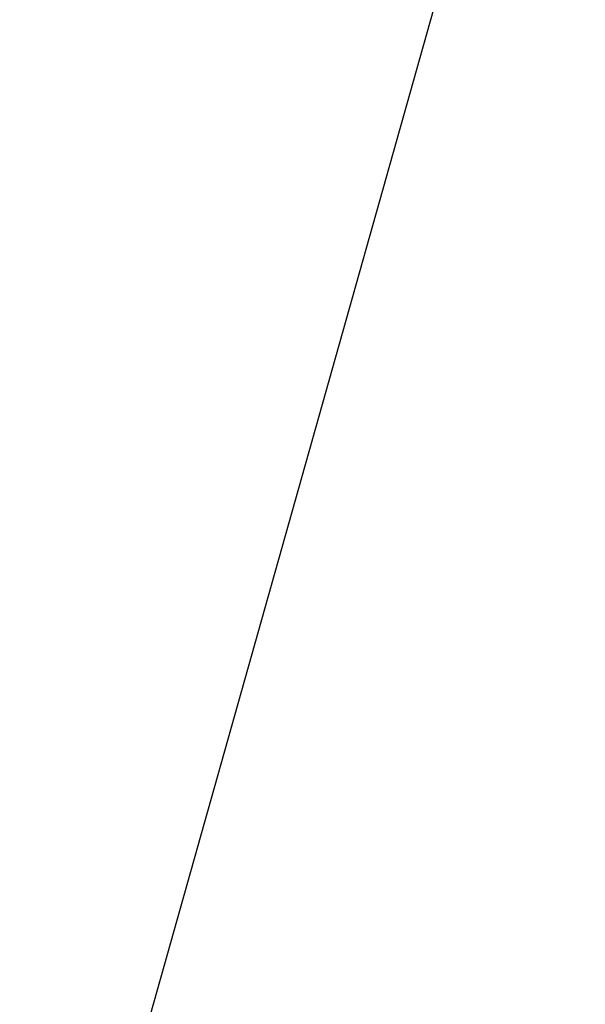
# Model space of a CAD drawing. Units: inches. Extents: x 3590 to 5167, y 65 to 1917.
# Tile 88 of 100: x 5052.5773 to 5052.8768, y 1788.0928 to 1788.6144. Entities that reach past the tile are written whole.
import ezdxf

# ---------------------------------------------------------------- set-up
doc = ezdxf.new("R2010")
doc.units = ezdxf.units.IN
for name, color, linetype, lineweight in [('A-ANNO-DIMS', 2, 'Continuous', 18), ('A-FLOR-PATT', 8, 'Continuous', 13), ('L-PLNT', 94, 'Continuous', 18)]:
    doc.layers.add(name, color=color, linetype=linetype, lineweight=lineweight)
doc.layers.add('DIENHOA', color=3, linetype='Continuous')
doc.styles.get("Standard").update_dxf_attribs({"font": 'arial.ttf'})
doc.dimstyles.new('ISO-25', dxfattribs={"dimtxt": 9, "dimasz": 2.5, "dimexe": 1.25, "dimexo": 0.625, "dimtad": 1, "dimdec": 1, "dimlunit": 3, "dimtxsty": 'Standard', "dimcen": 2.5, "dimadec": 0, "dimazin": 0, "dimtfac": 1, "dimtdec": 1, "dimtmove": 0, "dimatfit": 3, "dimfxl": 1, "dimarcsym": 0})

# ---------------------------------------------------------------- blocks, each defined once
blk = doc.blocks.new('Cay03_mb')
at = {"layer": 'DIENHOA'}
blk.add_line((96.72, 365.576), (75.598, 290.611), dxfattribs=at)
blk = doc.blocks.new('*D322')
at = {"layer": 'A-ANNO-DIMS', "color": 0, "lineweight": -2, "transparency": 16777216}
for p, q in [((5035.74373, 1766.18424), (5035.74373, 1761.19899)), ((5064.81203, 1766.18424), (5064.81203, 1761.19899)), ((5038.24373, 1762.44899), (5062.31203, 1762.44899)), ((5064.81203, 1762.44899), (5166.99109, 1762.44899))]:
    blk.add_line(p, q, dxfattribs=at)
at = {"layer": 'A-ANNO-DIMS', "color": 0, "transparency": 16777216}
for points in [[(5038.24373, 1762.86566), (5038.24373, 1762.03233), (5035.74373, 1762.44899)], [(5062.31203, 1762.86566), (5062.31203, 1762.03233), (5064.81203, 1762.44899)]]:
    blk.add_solid(points, dxfattribs=at)
at = {"layer": 'Defpoints', "color": 0, "transparency": 16777216}
for p in [(5035.74373, 1766.80924), (5064.81203, 1766.80924), (5064.81203, 1762.44899)]:
    blk.add_point(p, dxfattribs=at)
at = {"layer": 'A-ANNO-DIMS', "color": 0, "transparency": 16777216, "insert": (5117.15156, 1767.66915), "char_height": 9, "attachment_point": 5}
blk.add_mtext('PLANT 2\'-5" TYP.', dxfattribs=at)

msp = doc.modelspace()

# ---------------------------------------------------------------- hatches: boundary and pattern name
at = {"layer": 'A-FLOR-PATT', "transparency": 33554687}
h = msp.add_hatch(dxfattribs=at)
h.set_pattern_fill('AR-HBONE', color=256, scale=0.2)
h.set_pattern_definition([(45, (-588.972, 0), (0, 28.73682), [60.96, -20.32]), (135, (-574.604, 14.368), (3e-15, 28.73682), [60.96, -20.32])])
h.paths.add_polyline_path([(5071.27403, 1796.99898), (4933.27403, 1796.99898), (4933.27403, 1753.99898), (4962.77403, 1753.99898, -0.414214), (4928.77403, 1719.99898), (4933.27403, 1718.99898), (4933.27403, 1334.99898), (5071.27403, 1334.99898)])
h.paths.add_polyline_path([(4951.78002, 1521.0767), (4951.7151, 1521.0404), (4951.56345, 1520.89532)], flags=16)
h.paths.add_polyline_path([(4952.267, 1521.37645), (4952.1977, 1521.37111), (4952.19823, 1521.35558)], flags=0)
h.paths.add_polyline_path([(4967.05076, 1529.72832), (4965.23122, 1528.69444), (4963.41109, 1527.71401), (4961.75649, 1526.85081), (4963.58887, 1527.44938), (4964.03555, 1527.47802), (4962.9755, 1527.24902), (4961.76022, 1526.85203), (4959.79219, 1525.83406), (4958.00498, 1524.89483), (4956.24031, 1523.92961), (4954.50395, 1522.91854), (4954.1294, 1522.68163), (4953.36051, 1521.99688), (4953.36558, 1521.99754), (4953.605, 1522.06367), (4955.10605, 1522.76083), (4956.92108, 1523.43405), (4958.67784, 1523.91513), (4960.35834, 1524.20036), (4961.94456, 1524.28606), (4964.17144, 1524.10849), (4965.95752, 1523.30903), (4963.86273, 1522.97565), (4965.18742, 1522.49898), (4963.36614, 1522.49715), (4961.54526, 1522.48682), (4959.76359, 1522.46077), (4958.30414, 1522.4188), (4957.97356, 1522.38829), (4956.30692, 1522.2324), (4954.71821, 1522.07143), (4953.25077, 1521.89915), (4953.52509, 1521.62277), (4954.33087, 1521.37883), (4956.24263, 1521.22987), (4958.03913, 1520.92952), (4959.68424, 1520.48339), (4961.16007, 1519.89569), (4963.10699, 1518.80022), (4964.39286, 1517.32518), (4962.97306, 1517.72596), (4964.55841, 1516.66059), (4965.40664, 1515.70779), (4963.50733, 1516.32179), (4961.67995, 1517.0051), (4959.93478, 1517.74489), (4958.2821, 1518.52833), (4956.73216, 1519.34257), (4955.29527, 1520.17478), (4954.67155, 1520.57237), (4954.51279, 1520.6271), (4955.65848, 1519.31837), (4956.70263, 1517.98232), (4957.64403, 1516.64663), (4958.48545, 1515.33439), (4959.54998, 1513.52398), (4960.43768, 1511.76936), (4958.84107, 1513.6196), (4957.45175, 1515.3249), (4955.8186, 1517.45855), (4956.66537, 1515.44764), (4957.11109, 1513.92292), (4957.44681, 1511.71434), (4957.07641, 1509.79288), (4956.53757, 1511.1103), (4955.99231, 1512.56892), (4955.44448, 1514.12509), (4954.89794, 1515.73518), (4954.35653, 1517.35553), (4953.82412, 1518.94251), (4953.30455, 1520.45247), (4953.06452, 1521.11563), (4952.97143, 1521.14607), (4952.94932, 1521.08646), (4952.72981, 1520.19905), (4953.3698, 1518.02364), (4953.75708, 1516.37279), (4954.05124, 1514.76538), (4954.26449, 1513.22121), (4954.47124, 1511.13121), (4954.4971, 1510.40174), (4954.40903, 1511.76006), (4954.26449, 1513.22121), (4954.05124, 1514.76538), (4953.75708, 1516.37279), (4953.3698, 1518.02364), (4952.87718, 1519.69813), (4952.7161, 1520.1412), (4952.53301, 1519.05871), (4952.37428, 1517.78881), (4952.21925, 1516.31167), (4952.04598, 1514.59986), (4951.83253, 1512.62598), (4951.55697, 1510.36259), (4951.20331, 1512.16818), (4950.85168, 1514.33931), (4950.98529, 1516.37594), (4951.6596, 1518.28625), (4952.59261, 1520.48085), (4952.35664, 1521.1299), (4951.85502, 1520.32753), (4950.83901, 1518.90828), (4949.77675, 1517.58658), (4948.91554, 1516.61731), (4948.11099, 1515.2561), (4947.0891, 1513.55389), (4945.88937, 1511.61495), (4946.32587, 1513.40232), (4946.5624, 1514.24913), (4945.52771, 1513.32668), (4944.58105, 1512.53126), (4946.01774, 1514.50825), (4947.2044, 1516.04763), (4947.89331, 1517.31331), (4949.30686, 1518.76446), (4950.41417, 1519.76716), (4950.45131, 1519.80628), (4952.267, 1521.37645), (4951.64457, 1521.49317), (4950.40371, 1521.17954), (4948.04447, 1520.35868), (4946.11863, 1519.45198), (4944.57182, 1518.47484), (4943.34962, 1517.44265), (4941.99695, 1515.91971), (4941.66146, 1515.27475), (4942.81332, 1516.98973), (4944.57182, 1518.47484), (4946.11863, 1519.45198), (4948.04447, 1520.35868), (4950.40371, 1521.17954), (4951.64457, 1521.49317), (4949.64678, 1521.86781), (4948.59979, 1521.75633), (4947.12629, 1521.5699), (4945.42015, 1521.34763), (4943.44969, 1521.10462), (4941.18319, 1520.85596), (4942.86028, 1521.61265), (4943.87308, 1522.03014), (4942.95216, 1521.9093), (4941.40968, 1521.48512), (4939.54287, 1520.67019), (4938.96775, 1520.2255), (4940.73284, 1521.29899), (4942.95216, 1521.9093), (4943.70184, 1522.00767), (4945.89419, 1522.69998), (4947.56488, 1522.71399), (4948.92086, 1522.56573), (4951.13144, 1522.18271), (4950.97062, 1522.2969), (4948.12924, 1523.00563), (4946.03496, 1523.70671), (4944.23235, 1524.52143), (4942.70692, 1525.46111), (4941.44419, 1526.53707), (4940.42968, 1527.76062), (4939.6489, 1529.14306), (4941.42091, 1528.12232), (4943.14742, 1527.13248), (4944.84093, 1526.17457), (4946.51394, 1525.24959), (4948.17893, 1524.35855), (4948.36457, 1524.26336), (4946.47531, 1526.04459), (4945.18083, 1527.54042), (4944.19039, 1529.03339), (4943.49559, 1530.53985), (4943.27808, 1531.3597), (4942.49849, 1531.91903), (4943.11353, 1531.76249), (4942.95927, 1533.6586), (4944.13953, 1531.9886), (4944.61171, 1531.32339), (4946.20163, 1530.46341), (4947.48567, 1529.50925), (4948.79027, 1528.22649), (4950.36754, 1526.23746), (4949.48547, 1528.15549), (4948.85128, 1530.12254), (4948.49054, 1532.04127), (4948.38105, 1533.91822), (4948.50062, 1535.7599), (4948.82704, 1537.57284), (4949.41803, 1535.56526), (4949.95684, 1533.56932), (4950.46414, 1531.5861), (4950.96058, 1529.6167), (4951.3911, 1527.95448), (4951.72352, 1530.68689), (4952.20106, 1532.57994), (4952.88914, 1534.32964), (4953.77035, 1535.95123), (4954.82726, 1537.45995), (4954.52145, 1535.38966), (4954.27314, 1533.93684), (4955.57999, 1535.6627), (4956.74758, 1536.73859), (4956.15852, 1534.78029), (4955.58917, 1532.87334), (4955.04336, 1531.00581), (4954.52493, 1529.16576), (4954.03771, 1527.34127), (4953.63833, 1525.73298), (4953.61143, 1525.58564), (4953.39805, 1524.16565), (4953.38219, 1524.00887), (4954.06955, 1525.47563), (4954.91212, 1527.02173), (4956.13627, 1528.89351), (4957.84668, 1530.57701), (4959.37601, 1531.54014), (4958.25596, 1530.10398), (4957.14284, 1528.66291), (4956.06626, 1527.24305), (4955.05579, 1525.87054), (4954.14104, 1524.57149), (4953.35159, 1523.37204), (4953.31079, 1523.30299), (4953.27253, 1522.92478), (4953.26102, 1522.38213), (4954.1031, 1523.37273), (4954.63005, 1524.28376), (4955.96149, 1526.35767), (4957.23002, 1528.12969), (4958.42057, 1529.60864), (4960.03671, 1531.36792), (4961.3736, 1532.3752), (4962.1015, 1532.77), (4961.06994, 1531.06113), (4959.98733, 1529.43811), (4958.86851, 1527.90803), (4958.15046, 1527.00742), (4959.80291, 1528.00314), (4961.58854, 1528.79257), (4963.39087, 1529.32783), (4965.21118, 1529.63205)], flags=16)
h.paths.add_polyline_path([(4962.94387, 1523.18187), (4961.10714, 1523.42192), (4960.39205, 1523.36158), (4962.34964, 1523.33061)], flags=0)
h.paths.add_polyline_path([(5049.54129, 1584.55089), (5049.47636, 1584.51458), (5049.32471, 1584.3695)], flags=16)
h.paths.add_polyline_path([(5050.02827, 1584.85063), (5049.95897, 1584.84529), (5049.95949, 1584.82976)], flags=0)
h.paths.add_polyline_path([(5042.33308, 1581.94902), (5043.8799, 1582.92616), (5045.80573, 1583.83286), (5048.16498, 1584.65372), (5049.40583, 1584.96736), (5047.40804, 1585.34199), (5046.36106, 1585.23052), (5044.88755, 1585.04408), (5043.18142, 1584.82181), (5041.21095, 1584.5788), (5038.94446, 1584.33014), (5040.62155, 1585.08683), (5041.63434, 1585.50432), (5040.71343, 1585.38348), (5039.17095, 1584.9593), (5037.30414, 1584.14438), (5036.72901, 1583.69969), (5038.4941, 1584.77317), (5040.71343, 1585.38348), (5041.4631, 1585.48185), (5043.65545, 1586.17416), (5045.32615, 1586.18818), (5046.68212, 1586.03992), (5048.8927, 1585.6569), (5048.73188, 1585.77108), (5045.89051, 1586.47981), (5043.79622, 1587.18089), (5041.99361, 1587.99561), (5040.46818, 1588.9353), (5039.20546, 1590.01125), (5038.19095, 1591.2348), (5037.41016, 1592.61725), (5039.18217, 1591.5965), (5040.90868, 1590.60667), (5042.6022, 1589.64876), (5044.2752, 1588.72378), (5045.94019, 1587.83274), (5046.12584, 1587.73754), (5044.23658, 1589.51878), (5042.9421, 1591.01461), (5041.95166, 1592.50757), (5041.25685, 1594.01403), (5041.03935, 1594.83388), (5040.25976, 1595.39321), (5040.8748, 1595.23667), (5040.72054, 1597.13279), (5041.9008, 1595.46278), (5042.37297, 1594.79758), (5043.96289, 1593.93759), (5045.24694, 1592.98344), (5046.55153, 1591.70068), (5048.12881, 1589.71164), (5047.24673, 1591.62967), (5046.61254, 1593.59672), (5046.2518, 1595.51546), (5046.14232, 1597.3924), (5046.26189, 1599.23408), (5046.5883, 1601.04703), (5047.17929, 1599.03944), (5047.71811, 1597.0435), (5048.22541, 1595.06028), (5048.72184, 1593.09089), (5049.15237, 1591.42866), (5049.48478, 1594.16107), (5049.96233, 1596.05412), (5050.65041, 1597.80382), (5051.53161, 1599.42541), (5052.58852, 1600.93414), (5052.28271, 1598.86384), (5052.03441, 1597.41102), (5053.34126, 1599.13689), (5054.50884, 1600.21277), (5053.91979, 1598.25447), (5053.35044, 1596.34752), (5052.80463, 1594.47999), (5052.2862, 1592.63995), (5051.79898, 1590.81546), (5051.39959, 1589.20716), (5051.3727, 1589.05983), (5051.15931, 1587.63984), (5051.14346, 1587.48305), (5051.83082, 1588.94982), (5052.67339, 1590.49592), (5053.89754, 1592.3677), (5055.60794, 1594.05119), (5057.13728, 1595.01432), (5056.01722, 1593.57817), (5054.90411, 1592.1371), (5053.82752, 1590.71724), (5052.81705, 1589.34472), (5051.9023, 1588.04567), (5051.11286, 1586.84622), (5051.07205, 1586.77718), (5051.03379, 1586.39896), (5051.02228, 1585.85631), (5051.86437, 1586.84692), (5052.39131, 1587.75794), (5053.72275, 1589.83185), (5054.99128, 1591.60387), (5056.18183, 1593.08282), (5057.79798, 1594.84211), (5059.13486, 1595.84938), (5059.86276, 1596.24419), (5058.83121, 1594.53531), (5057.7486, 1592.9123), (5056.62978, 1591.38221), (5055.91173, 1590.4816), (5057.56418, 1591.47732), (5059.34981, 1592.26675), (5061.15214, 1592.80202), (5062.97245, 1593.10624), (5064.81203, 1593.20251), (5062.99248, 1592.16863), (5061.17235, 1591.18819), (5059.51775, 1590.325), (5061.35014, 1590.92356), (5061.79682, 1590.95221), (5060.73676, 1590.7232), (5059.52148, 1590.32622), (5057.55345, 1589.30825), (5055.76625, 1588.36901), (5054.00157, 1587.40379), (5052.26521, 1586.39273), (5051.89067, 1586.15581), (5051.12177, 1585.47106), (5051.12684, 1585.47172), (5051.36627, 1585.53786), (5052.86732, 1586.23502), (5054.68234, 1586.90824), (5056.4391, 1587.38931), (5058.1196, 1587.67454), (5059.70582, 1587.76024), (5061.93271, 1587.58268), (5063.71878, 1586.78321), (5061.62399, 1586.44983), (5062.94869, 1585.97317), (5061.12741, 1585.97133), (5059.30653, 1585.961), (5057.52486, 1585.93496), (5056.06541, 1585.89299), (5055.73482, 1585.86247), (5054.06819, 1585.70658), (5052.47947, 1585.54561), (5051.01204, 1585.37333), (5051.28635, 1585.09695), (5052.09214, 1584.85301), (5054.00389, 1584.70406), (5055.8004, 1584.4037), (5057.44551, 1583.95757), (5058.92133, 1583.36987), (5060.86825, 1582.27441), (5062.15413, 1580.79937), (5060.73433, 1581.20015), (5062.31967, 1580.13477), (5063.1679, 1579.18198), (5061.2686, 1579.79597), (5059.44122, 1580.47928), (5057.69605, 1581.21908), (5056.04336, 1582.00251), (5054.49343, 1582.81675), (5053.05653, 1583.64897), (5052.43281, 1584.04656), (5052.27405, 1584.10128), (5053.41974, 1582.79255), (5054.4639, 1581.4565), (5055.40529, 1580.12081), (5056.24672, 1578.80858), (5057.31125, 1576.99816), (5058.19895, 1575.24354), (5056.60234, 1577.09378), (5055.21301, 1578.79908), (5053.57987, 1580.93274), (5054.42664, 1578.92183), (5054.87235, 1577.3971), (5055.20808, 1575.18852), (5054.83767, 1573.26706), (5054.29883, 1574.58448), (5053.75357, 1576.0431), (5053.20575, 1577.59927), (5052.6592, 1579.20936), (5052.1178, 1580.82971), (5051.58538, 1582.41669), (5051.06582, 1583.92666), (5050.82578, 1584.58981), (5050.7327, 1584.62025), (5050.71058, 1584.56064), (5050.49108, 1583.67323), (5051.13107, 1581.49782), (5051.51835, 1579.84698), (5051.8125, 1578.23957), (5052.02575, 1576.69539), (5052.23251, 1574.6054), (5052.25836, 1573.87593), (5052.1703, 1575.23424), (5052.02575, 1576.69539), (5051.8125, 1578.23957), (5051.51835, 1579.84698), (5051.13107, 1581.49782), (5050.63844, 1583.17231), (5050.47736, 1583.61538), (5050.29428, 1582.53289), (5050.13554, 1581.26299), (5049.98051, 1579.78585), (5049.80724, 1578.07405), (5049.59379, 1576.10016), (5049.31823, 1573.83678), (5048.96458, 1575.64237), (5048.61294, 1577.8135), (5048.74656, 1579.85012), (5049.42086, 1581.76043), (5050.35388, 1583.95503), (5050.1179, 1584.60408), (5049.61629, 1583.80172), (5048.60027, 1582.38246), (5047.53801, 1581.06076), (5046.67681, 1580.09149), (5045.87225, 1578.73029), (5044.85036, 1577.02808), (5043.65063, 1575.08913), (5044.08713, 1576.8765), (5044.32366, 1577.72331), (5043.28898, 1576.80086), (5042.34232, 1576.00545), (5043.779, 1577.98243), (5044.96566, 1579.52182), (5045.65457, 1580.78749), (5047.06813, 1582.23865), (5048.17543, 1583.24134), (5048.21258, 1583.28047), (5050.02827, 1584.85063), (5049.40583, 1584.96736), (5048.16498, 1584.65372), (5045.80573, 1583.83286), (5043.8799, 1582.92616), (5042.33308, 1581.94902), (5041.11088, 1580.91684), (5039.75821, 1579.39389), (5039.42272, 1578.74894), (5040.57458, 1580.46391)], flags=16)
h.paths.add_polyline_path([(4954.79872, 1533.12029), (4954.26249, 1532.07935), (4953.83112, 1530.93464), (4953.50472, 1529.63602), (4953.28338, 1528.13331), (4953.16721, 1526.37637), (4953.15631, 1524.31504), (4953.27669, 1521.23629), (4952.80168, 1521.84177), (4951.55695, 1521.99789), (4950.97575, 1521.9613), (4952.66059, 1521.94097), (4952.80168, 1521.84177), (4953.15249, 1523.59258), (4953.16721, 1526.37637), (4953.28338, 1528.13331), (4953.60929, 1530.34598), (4954.45558, 1532.59174)], flags=0)
h.paths.add_polyline_path([(5050.56294, 1585.31596), (5049.31822, 1585.47208), (5048.73702, 1585.43548), (5050.42186, 1585.41516), (5050.56294, 1585.31596), (5050.91375, 1587.06676), (5050.92848, 1589.85056), (5051.04465, 1591.6075), (5051.37055, 1593.82017), (5052.21684, 1596.06593), (5052.55999, 1596.59447), (5052.02375, 1595.55353), (5051.59238, 1594.40883), (5051.26598, 1593.1102), (5051.04465, 1591.6075), (5050.92848, 1589.85056), (5050.91757, 1587.78922), (5051.03795, 1584.71048)], flags=0)
h.paths.add_polyline_path([(5058.15332, 1586.83576), (5060.11091, 1586.80479), (5060.70514, 1586.65605), (5058.8684, 1586.8961)], flags=0)
h.paths.add_polyline_path([(5049.54129, 1430.93611), (5049.47636, 1430.8998), (5049.32471, 1430.75472)], flags=16)
h.paths.add_polyline_path([(5050.02827, 1431.23585), (5049.95897, 1431.23051), (5049.95949, 1431.21498)], flags=0)
h.paths.add_polyline_path([(5046.5883, 1447.43225), (5047.17929, 1445.42467), (5047.71811, 1443.42872), (5048.22541, 1441.4455), (5048.72184, 1439.47611), (5049.15237, 1437.81388), (5049.48478, 1440.5463), (5049.96233, 1442.43934), (5050.65041, 1444.18904), (5051.53161, 1445.81063), (5052.58852, 1447.31936), (5052.28271, 1445.24906), (5052.03441, 1443.79624), (5053.34126, 1445.52211), (5054.50884, 1446.59799), (5053.91979, 1444.63969), (5053.35044, 1442.73274), (5052.80463, 1440.86521), (5052.2862, 1439.02517), (5051.79898, 1437.20068), (5051.39959, 1435.59238), (5051.3727, 1435.44505), (5051.15931, 1434.02506), (5051.14346, 1433.86828), (5051.83082, 1435.33504), (5052.67339, 1436.88114), (5053.89754, 1438.75292), (5055.60794, 1440.43641), (5057.13728, 1441.39954), (5056.01722, 1439.96339), (5054.90411, 1438.52232), (5053.82752, 1437.10246), (5052.81705, 1435.72994), (5051.9023, 1434.4309), (5051.11286, 1433.23145), (5051.07205, 1433.1624), (5051.03379, 1432.78418), (5051.02228, 1432.24153), (5051.86437, 1433.23214), (5052.39131, 1434.14316), (5053.72275, 1436.21707), (5054.99128, 1437.98909), (5056.18183, 1439.46805), (5057.79798, 1441.22733), (5059.13486, 1442.23461), (5059.86276, 1442.62941), (5058.83121, 1440.92053), (5057.7486, 1439.29752), (5056.62978, 1437.76743), (5055.91173, 1436.86682), (5057.56418, 1437.86255), (5059.34981, 1438.65197), (5061.15214, 1439.18724), (5062.97245, 1439.49146), (5064.81203, 1439.58773), (5062.99248, 1438.55385), (5061.17235, 1437.57342), (5059.51775, 1436.71022), (5061.35014, 1437.30879), (5061.79682, 1437.33743), (5060.73676, 1437.10842), (5059.52148, 1436.71144), (5057.55345, 1435.69347), (5055.76625, 1434.75423), (5054.00157, 1433.78901), (5052.26521, 1432.77795), (5051.89067, 1432.54103), (5051.12177, 1431.85628), (5051.12684, 1431.85694), (5051.36627, 1431.92308), (5052.86732, 1432.62024), (5054.68234, 1433.29346), (5056.4391, 1433.77453), (5058.1196, 1434.05976), (5059.70582, 1434.14546), (5061.93271, 1433.9679), (5063.71878, 1433.16843), (5061.62399, 1432.83505), (5062.94869, 1432.35839), (5061.12741, 1432.35655), (5059.30653, 1432.34623), (5057.52486, 1432.32018), (5056.06541, 1432.27821), (5055.73482, 1432.24769), (5054.06819, 1432.09181), (5052.47947, 1431.93083), (5051.01204, 1431.75856), (5051.28635, 1431.48218), (5052.09214, 1431.23823), (5054.00389, 1431.08928), (5055.8004, 1430.78892), (5057.44551, 1430.34279), (5058.92133, 1429.75509), (5060.86825, 1428.65963), (5062.15413, 1427.18459), (5060.73433, 1427.58537), (5062.31967, 1426.52), (5063.1679, 1425.5672), (5061.2686, 1426.18119), (5059.44122, 1426.86451), (5057.69605, 1427.6043), (5056.04336, 1428.38773), (5054.49343, 1429.20197), (5053.05653, 1430.03419), (5052.43281, 1430.43178), (5052.27405, 1430.48651), (5053.41974, 1429.17777), (5054.4639, 1427.84172), (5055.40529, 1426.50603), (5056.24672, 1425.1938), (5057.31125, 1423.38338), (5058.19895, 1421.62877), (5056.60234, 1423.479), (5055.21301, 1425.1843), (5053.57987, 1427.31796), (5054.42664, 1425.30705), (5054.87235, 1423.78233), (5055.20808, 1421.57374), (5054.83767, 1419.65228), (5054.29883, 1420.9697), (5053.75357, 1422.42832), (5053.20575, 1423.9845), (5052.6592, 1425.59458), (5052.1178, 1427.21493), (5051.58538, 1428.80191), (5051.06582, 1430.31188), (5050.82578, 1430.97503), (5050.7327, 1431.00547), (5050.71058, 1430.94586), (5050.49108, 1430.05845), (5051.13107, 1427.88305), (5051.51835, 1426.2322), (5051.8125, 1424.62479), (5052.02575, 1423.08061), (5052.23251, 1420.99062), (5052.25836, 1420.26115), (5052.1703, 1421.61947), (5052.02575, 1423.08061), (5051.8125, 1424.62479), (5051.51835, 1426.2322), (5051.13107, 1427.88305), (5050.63844, 1429.55753), (5050.47736, 1430.0006), (5050.29428, 1428.91811), (5050.13554, 1427.64821), (5049.98051, 1426.17107), (5049.80724, 1424.45927), (5049.59379, 1422.48539), (5049.31823, 1420.222), (5048.96458, 1422.02759), (5048.61294, 1424.19872), (5048.74656, 1426.23534), (5049.42086, 1428.14565), (5050.35388, 1430.34025), (5050.1179, 1430.98931), (5049.61629, 1430.18694), (5048.60027, 1428.76768), (5047.53801, 1427.44598), (5046.67681, 1426.47671), (5045.87225, 1425.11551), (5044.85036, 1423.4133), (5043.65063, 1421.47435), (5044.08713, 1423.26172), (5044.32366, 1424.10854), (5043.28898, 1423.18608), (5042.34232, 1422.39067), (5043.779, 1424.36765), (5044.96566, 1425.90704), (5045.65457, 1427.17272), (5047.06813, 1428.62387), (5048.17543, 1429.62657), (5048.21258, 1429.66569), (5050.02827, 1431.23585), (5049.40583, 1431.35258), (5048.16498, 1431.03894), (5045.80573, 1430.21809), (5043.8799, 1429.31139), (5042.33308, 1428.33424), (5041.11088, 1427.30206), (5039.75821, 1425.77911), (5039.42272, 1425.13416), (5040.57458, 1426.84914), (5042.33308, 1428.33424), (5043.8799, 1429.31139), (5045.80573, 1430.21809), (5048.16498, 1431.03894), (5049.40583, 1431.35258), (5047.40804, 1431.72722), (5046.36106, 1431.61574), (5044.88755, 1431.42931), (5043.18142, 1431.20704), (5041.21095, 1430.96402), (5038.94446, 1430.71536), (5040.62155, 1431.47205), (5041.63434, 1431.88954), (5040.71343, 1431.76871), (5039.17095, 1431.34453), (5037.30414, 1430.5296), (5036.72901, 1430.08491), (5038.4941, 1431.1584), (5040.71343, 1431.76871), (5041.4631, 1431.86707), (5043.65545, 1432.55939), (5045.32615, 1432.5734), (5046.68212, 1432.42514), (5048.8927, 1432.04212), (5048.73188, 1432.1563), (5045.89051, 1432.86503), (5043.79622, 1433.56611), (5041.99361, 1434.38083), (5040.46818, 1435.32052), (5039.20546, 1436.39648), (5038.19095, 1437.62002), (5037.41016, 1439.00247), (5039.18217, 1437.98172), (5040.90868, 1436.99189), (5042.6022, 1436.03398), (5044.2752, 1435.109), (5045.94019, 1434.21796), (5046.12584, 1434.12276), (5044.23658, 1435.904), (5042.9421, 1437.39983), (5041.95166, 1438.8928), (5041.25685, 1440.39925), (5041.03935, 1441.2191), (5040.25976, 1441.77844), (5040.8748, 1441.62189), (5040.72054, 1443.51801), (5041.9008, 1441.848), (5042.37297, 1441.1828), (5043.96289, 1440.32282), (5045.24694, 1439.36866), (5046.55153, 1438.0859), (5048.12881, 1436.09686), (5047.24673, 1438.01489), (5046.61254, 1439.98195), (5046.2518, 1441.90068), (5046.14232, 1443.77762), (5046.26189, 1445.6193)], flags=16)
h.paths.add_polyline_path([(5052.38176, 1444.25496), (5051.62263, 1442.77987), (5052.02375, 1441.93875), (5052.55999, 1442.9797)], flags=0)
h.paths.add_polyline_path([(5050.56294, 1431.70118), (5049.31822, 1431.8573), (5048.73702, 1431.82071), (5050.42186, 1431.80038)], flags=0)
h.paths.add_polyline_path([(5058.15332, 1433.22098), (5060.11091, 1433.19001), (5060.70514, 1433.04127), (5058.8684, 1433.28132)], flags=0)
h.paths.add_polyline_path([(5049.54129, 1352.28535), (5049.47636, 1352.24904), (5049.32471, 1352.10396)], flags=16)
h.paths.add_polyline_path([(5050.02827, 1352.58509), (5049.95897, 1352.57975), (5049.95949, 1352.56422)], flags=0)
h.paths.add_polyline_path([(5046.5883, 1368.78149), (5047.17929, 1366.7739), (5047.71811, 1364.77796), (5048.22541, 1362.79474), (5048.72184, 1360.82534), (5049.15237, 1359.16312), (5049.48478, 1361.89553), (5049.96233, 1363.78858), (5050.65041, 1365.53828), (5051.53161, 1367.15987), (5052.58852, 1368.6686), (5052.28271, 1366.5983), (5052.03441, 1365.14548), (5053.34126, 1366.87135), (5054.50884, 1367.94723), (5053.91979, 1365.98893), (5053.35044, 1364.08198), (5052.80463, 1362.21445), (5052.2862, 1360.37441), (5051.79898, 1358.54992), (5051.39959, 1356.94162), (5051.3727, 1356.79428), (5051.15931, 1355.37429), (5051.14346, 1355.21751), (5051.83082, 1356.68428), (5052.67339, 1358.23037), (5053.89754, 1360.10216), (5055.60794, 1361.78565), (5057.13728, 1362.74878), (5056.01722, 1361.31262), (5054.90411, 1359.87155), (5053.82752, 1358.4517), (5052.81705, 1357.07918), (5051.9023, 1355.78013), (5051.11286, 1354.58068), (5051.07205, 1354.51164), (5051.03379, 1354.13342), (5051.02228, 1353.59077), (5051.86437, 1354.58137), (5052.39131, 1355.4924), (5053.72275, 1357.56631), (5054.99128, 1359.33833), (5056.18183, 1360.81728), (5057.79798, 1362.57656), (5059.13486, 1363.58384), (5059.86276, 1363.97864), (5058.83121, 1362.26977), (5057.7486, 1360.64675), (5056.62978, 1359.11667), (5055.91173, 1358.21606), (5057.56418, 1359.21178), (5059.34981, 1360.00121), (5061.15214, 1360.53648), (5062.97245, 1360.84069), (5064.81203, 1360.93697), (5062.99248, 1359.90308), (5061.17235, 1358.92265), (5059.51775, 1358.05946), (5061.35014, 1358.65802), (5061.79682, 1358.68666), (5060.73676, 1358.45766), (5059.52148, 1358.06068), (5057.55345, 1357.0427), (5055.76625, 1356.10347), (5054.00157, 1355.13825), (5052.26521, 1354.12718), (5051.89067, 1353.89027), (5051.12177, 1353.20552), (5051.12684, 1353.20618), (5051.36627, 1353.27231), (5052.86732, 1353.96947), (5054.68234, 1354.6427), (5056.4391, 1355.12377), (5058.1196, 1355.409), (5059.70582, 1355.4947), (5061.93271, 1355.31713), (5063.71878, 1354.51767), (5061.62399, 1354.18429), (5062.94869, 1353.70763), (5061.12741, 1353.70579), (5059.30653, 1353.69546), (5057.52486, 1353.66942), (5056.06541, 1353.62744), (5055.73482, 1353.59693), (5054.06819, 1353.44104), (5052.47947, 1353.28007), (5051.01204, 1353.10779), (5051.28635, 1352.83141), (5052.09214, 1352.58747), (5054.00389, 1352.43852), (5055.8004, 1352.13816), (5057.44551, 1351.69203), (5058.92133, 1351.10433), (5060.86825, 1350.00887), (5062.15413, 1348.53382), (5060.73433, 1348.9346), (5062.31967, 1347.86923), (5063.1679, 1346.91643), (5061.2686, 1347.53043), (5059.44122, 1348.21374), (5057.69605, 1348.95353), (5056.04336, 1349.73697), (5054.49343, 1350.55121), (5053.05653, 1351.38342), (5052.43281, 1351.78101), (5052.27405, 1351.83574), (5053.41974, 1350.52701), (5054.4639, 1349.19096), (5055.40529, 1347.85527), (5056.24672, 1346.54303), (5057.31125, 1344.73262), (5058.19895, 1342.978), (5056.60234, 1344.82824), (5055.21301, 1346.53354), (5053.57987, 1348.6672), (5054.42664, 1346.65629), (5054.87235, 1345.13156), (5055.20808, 1342.92298), (5054.83767, 1341.00152), (5054.29883, 1342.31894), (5053.75357, 1343.77756), (5053.20575, 1345.33373), (5052.6592, 1346.94382), (5052.1178, 1348.56417), (5051.58538, 1350.15115), (5051.06582, 1351.66111), (5050.82578, 1352.32427), (5050.7327, 1352.35471), (5050.71058, 1352.2951), (5050.49108, 1351.40769), (5051.13107, 1349.23228), (5051.51835, 1347.58144), (5051.8125, 1345.97403), (5052.02575, 1344.42985), (5052.23251, 1342.33986), (5052.25836, 1341.61039), (5052.1703, 1342.9687), (5052.02575, 1344.42985), (5051.8125, 1345.97403), (5051.51835, 1347.58144), (5051.13107, 1349.23228), (5050.63844, 1350.90677), (5050.47736, 1351.34984), (5050.29428, 1350.26735), (5050.13554, 1348.99745), (5049.98051, 1347.52031), (5049.80724, 1345.80851), (5049.59379, 1343.83462), (5049.31823, 1341.57124), (5048.96458, 1343.37683), (5048.61294, 1345.54796), (5048.74656, 1347.58458), (5049.42086, 1349.49489), (5050.35388, 1351.68949), (5050.1179, 1352.33854), (5049.61629, 1351.53617), (5048.60027, 1350.11692), (5047.53801, 1348.79522), (5046.67681, 1347.82595), (5045.87225, 1346.46475), (5044.85036, 1344.76253), (5043.65063, 1342.82359), (5044.08713, 1344.61096), (5044.32366, 1345.45777), (5043.28898, 1344.53532), (5042.34232, 1343.7399), (5043.779, 1345.71689), (5044.96566, 1347.25627), (5045.65457, 1348.52195), (5047.06813, 1349.9731), (5048.17543, 1350.9758), (5048.21258, 1351.01493), (5050.02827, 1352.58509), (5049.40583, 1352.70181), (5048.16498, 1352.38818), (5045.80573, 1351.56732), (5043.8799, 1350.66062), (5042.33308, 1349.68348), (5041.11088, 1348.65129), (5039.75821, 1347.12835), (5039.42272, 1346.4834), (5040.57458, 1348.19837), (5042.33308, 1349.68348), (5043.8799, 1350.66062), (5045.80573, 1351.56732), (5048.16498, 1352.38818), (5049.40583, 1352.70181), (5047.40804, 1353.07645), (5046.36106, 1352.96498), (5044.88755, 1352.77854), (5043.18142, 1352.55627), (5041.21095, 1352.31326), (5038.94446, 1352.0646), (5040.62155, 1352.82129), (5041.63434, 1353.23878), (5040.71343, 1353.11794), (5039.17095, 1352.69376), (5037.30414, 1351.87884), (5036.72901, 1351.43415), (5038.4941, 1352.50763), (5040.71343, 1353.11794), (5041.4631, 1353.21631), (5043.65545, 1353.90862), (5045.32615, 1353.92263), (5046.68212, 1353.77438), (5048.8927, 1353.39136), (5048.73188, 1353.50554), (5045.89051, 1354.21427), (5043.79622, 1354.91535), (5041.99361, 1355.73007), (5040.46818, 1356.66975), (5039.20546, 1357.74571), (5038.19095, 1358.96926), (5037.41016, 1360.35171), (5039.18217, 1359.33096), (5040.90868, 1358.34112), (5042.6022, 1357.38321), (5044.2752, 1356.45824), (5045.94019, 1355.5672), (5046.12584, 1355.472), (5044.23658, 1357.25323), (5042.9421, 1358.74906), (5041.95166, 1360.24203), (5041.25685, 1361.74849), (5041.03935, 1362.56834), (5040.25976, 1363.12767), (5040.8748, 1362.97113), (5040.72054, 1364.86725), (5041.9008, 1363.19724), (5042.37297, 1362.53203), (5043.96289, 1361.67205), (5045.24694, 1360.7179), (5046.55153, 1359.43513), (5048.12881, 1357.4461), (5047.24673, 1359.36413), (5046.61254, 1361.33118), (5046.2518, 1363.24992), (5046.14232, 1365.12686), (5046.26189, 1366.96854)], flags=16)
h.paths.add_polyline_path([(5052.38176, 1365.6042), (5051.62263, 1364.12911), (5052.02375, 1363.28799), (5052.55999, 1364.32893)], flags=0)
h.paths.add_polyline_path([(4951.78002, 1698.04081), (4951.7151, 1698.0045), (4951.56345, 1697.85942)], flags=16)
h.paths.add_polyline_path([(4952.267, 1698.34055), (4952.1977, 1698.33521), (4952.19823, 1698.31968)], flags=0)
h.paths.add_polyline_path([(4957.07641, 1686.75698), (4956.53757, 1688.0744), (4955.99231, 1689.53302), (4955.44448, 1691.08919), (4954.89794, 1692.69928), (4954.35653, 1694.31963), (4953.82412, 1695.90661), (4953.30455, 1697.41658), (4953.06452, 1698.07973), (4952.97143, 1698.11017), (4952.94932, 1698.05056), (4952.72981, 1697.16315), (4953.3698, 1694.98774), (4953.75708, 1693.3369), (4954.05124, 1691.72949), (4954.26449, 1690.18531), (4954.47124, 1688.09532), (4954.4971, 1687.36585), (4954.40903, 1688.72416), (4954.26449, 1690.18531), (4954.05124, 1691.72949), (4953.75708, 1693.3369), (4953.3698, 1694.98774), (4952.87718, 1696.66223), (4952.7161, 1697.1053), (4952.53301, 1696.02281), (4952.37428, 1694.75291), (4952.21925, 1693.27577), (4952.04598, 1691.56397), (4951.83253, 1689.59008), (4951.55697, 1687.3267), (4951.20331, 1689.13229), (4950.85168, 1691.30342), (4950.98529, 1693.34004), (4951.6596, 1695.25035), (4952.59261, 1697.44495), (4952.35664, 1698.09401), (4951.85502, 1697.29164), (4950.83901, 1695.87238), (4949.77675, 1694.55068), (4948.91554, 1693.58141), (4948.11099, 1692.22021), (4947.0891, 1690.518), (4945.88937, 1688.57905), (4946.32587, 1690.36642), (4946.5624, 1691.21323), (4945.52771, 1690.29078), (4944.58105, 1689.49537), (4946.01774, 1691.47235), (4947.2044, 1693.01174), (4947.89331, 1694.27741), (4949.30686, 1695.72857), (4950.41417, 1696.73127), (4950.45131, 1696.77039), (4952.267, 1698.34055), (4951.64457, 1698.45728), (4950.40371, 1698.14364), (4948.04447, 1697.32278), (4946.11863, 1696.41608), (4944.57182, 1695.43894), (4943.34962, 1694.40676), (4941.99695, 1692.88381), (4941.66146, 1692.23886), (4942.81332, 1693.95383), (4944.57182, 1695.43894), (4946.11863, 1696.41608), (4948.04447, 1697.32278), (4950.40371, 1698.14364), (4951.64457, 1698.45728), (4949.64678, 1698.83191), (4948.59979, 1698.72044), (4947.12629, 1698.53401), (4945.42015, 1698.31174), (4943.44969, 1698.06872), (4941.18319, 1697.82006), (4942.86028, 1698.57675), (4943.87308, 1698.99424), (4942.95216, 1698.8734), (4941.40968, 1698.44922), (4939.54287, 1697.6343), (4938.96775, 1697.18961), (4940.73284, 1698.26309), (4942.95216, 1698.8734), (4943.70184, 1698.97177), (4945.89419, 1699.66409), (4947.56488, 1699.6781), (4948.92086, 1699.52984), (4951.13144, 1699.14682), (4950.97062, 1699.261), (4948.12924, 1699.96973), (4946.03496, 1700.67081), (4944.23235, 1701.48553), (4942.70692, 1702.42522), (4941.44419, 1703.50117), (4940.42968, 1704.72472), (4939.6489, 1706.10717), (4941.42091, 1705.08642), (4943.14742, 1704.09659), (4944.84093, 1703.13868), (4946.51394, 1702.2137), (4948.17893, 1701.32266), (4948.36457, 1701.22746), (4946.47531, 1703.0087), (4945.18083, 1704.50453), (4944.19039, 1705.9975), (4943.49559, 1707.50395), (4943.27808, 1708.3238), (4942.49849, 1708.88314), (4943.11353, 1708.72659), (4942.95927, 1710.62271), (4944.13953, 1708.9527), (4944.61171, 1708.2875), (4946.20163, 1707.42751), (4947.48567, 1706.47336), (4948.79027, 1705.1906), (4950.36754, 1703.20156), (4949.48547, 1705.11959), (4948.85128, 1707.08664), (4948.49054, 1709.00538), (4948.38105, 1710.88232), (4948.50062, 1712.724), (4948.82704, 1714.53695), (4949.41803, 1712.52937), (4949.95684, 1710.53342), (4950.46414, 1708.5502), (4950.96058, 1706.58081), (4951.3911, 1704.91858), (4951.72352, 1707.65099), (4952.20106, 1709.54404), (4952.88914, 1711.29374), (4953.77035, 1712.91533), (4954.82726, 1714.42406), (4954.52145, 1712.35376), (4954.27314, 1710.90094), (4955.57999, 1712.62681), (4956.74758, 1713.70269), (4956.15852, 1711.74439), (4955.58917, 1709.83744), (4955.04336, 1707.96991), (4954.52493, 1706.12987), (4954.03771, 1704.30538), (4953.63833, 1702.69708), (4953.61143, 1702.54975), (4953.39805, 1701.12976), (4953.38219, 1700.97297), (4954.06955, 1702.43974), (4954.91212, 1703.98584), (4956.13627, 1705.85762), (4957.84668, 1707.54111), (4959.37601, 1708.50424), (4958.25596, 1707.06809), (4957.14284, 1705.62702), (4956.06626, 1704.20716), (4955.05579, 1702.83464), (4954.14104, 1701.53559), (4953.35159, 1700.33614), (4953.31079, 1700.2671), (4953.27253, 1699.88888), (4953.26102, 1699.34623), (4954.1031, 1700.33684), (4954.63005, 1701.24786), (4955.96149, 1703.32177), (4957.23002, 1705.09379), (4958.42057, 1706.57274), (4960.03671, 1708.33203), (4961.3736, 1709.33931), (4962.1015, 1709.73411), (4961.06994, 1708.02523), (4959.98733, 1706.40222), (4958.86851, 1704.87213), (4958.15046, 1703.97152), (4959.80291, 1704.96725), (4961.58854, 1705.75667), (4963.39087, 1706.29194), (4965.21118, 1706.59616), (4967.05076, 1706.69243), (4965.23122, 1705.65855), (4963.41109, 1704.67811), (4961.75649, 1703.81492), (4963.58887, 1704.41349), (4964.03555, 1704.44213), (4962.9755, 1704.21312), (4961.76022, 1703.81614), (4959.79219, 1702.79817), (4958.00498, 1701.85893), (4956.24031, 1700.89371), (4954.50395, 1699.88265), (4954.1294, 1699.64573), (4953.36051, 1698.96098), (4953.36558, 1698.96164), (4953.605, 1699.02778), (4955.10605, 1699.72494), (4956.92108, 1700.39816), (4958.67784, 1700.87923), (4960.35834, 1701.16446), (4961.94456, 1701.25016), (4964.17144, 1701.0726), (4965.95752, 1700.27313), (4963.86273, 1699.93975), (4965.18742, 1699.46309), (4963.36614, 1699.46125), (4961.54526, 1699.45092), (4959.76359, 1699.42488), (4958.30414, 1699.38291), (4957.97356, 1699.35239), (4956.30692, 1699.1965), (4954.71821, 1699.03553), (4953.25077, 1698.86326), (4953.52509, 1698.58688), (4954.33087, 1698.34293), (4956.24263, 1698.19398), (4958.03913, 1697.89362), (4959.68424, 1697.44749), (4961.16007, 1696.85979), (4963.10699, 1695.76433), (4964.39286, 1694.28929), (4962.97306, 1694.69007), (4964.55841, 1693.6247), (4965.40664, 1692.6719), (4963.50733, 1693.28589), (4961.67995, 1693.9692), (4959.93478, 1694.709), (4958.2821, 1695.49243), (4956.73216, 1696.30667), (4955.29527, 1697.13889), (4954.67155, 1697.53648), (4954.51279, 1697.5912), (4955.65848, 1696.28247), (4956.70263, 1694.94642), (4957.64403, 1693.61073), (4958.48545, 1692.2985), (4959.54998, 1690.48808), (4960.43768, 1688.73346), (4958.84107, 1690.5837), (4957.45175, 1692.289), (4955.8186, 1694.42266), (4956.66537, 1692.41175), (4957.11109, 1690.88702), (4957.44681, 1688.67844)], flags=16)
h.paths.add_polyline_path([(5050.56294, 1353.05042), (5049.31822, 1353.20654), (5048.73702, 1353.16994), (5050.42186, 1353.14961)], flags=0)
h.paths.add_polyline_path([(4951.78002, 1351.48609), (4951.7151, 1351.44979), (4951.56345, 1351.30471)], flags=16)
h.paths.add_polyline_path([(4952.267, 1351.78584), (4952.1977, 1351.7805), (4952.19823, 1351.76497)], flags=0)
h.paths.add_polyline_path([(4954.82726, 1367.86934), (4954.52145, 1365.79905), (4954.27314, 1364.34623), (4955.57999, 1366.07209), (4956.74758, 1367.14798), (4956.15852, 1365.18968), (4955.58917, 1363.28273), (4955.04336, 1361.4152), (4954.52493, 1359.57515), (4954.03771, 1357.75066), (4953.63833, 1356.14237), (4953.61143, 1355.99503), (4953.39805, 1354.57504), (4953.38219, 1354.41826), (4954.06955, 1355.88503), (4954.91212, 1357.43112), (4956.13627, 1359.3029), (4957.84668, 1360.9864), (4959.37601, 1361.94953), (4958.25596, 1360.51337), (4957.14284, 1359.0723), (4956.06626, 1357.65245), (4955.05579, 1356.27993), (4954.14104, 1354.98088), (4953.35159, 1353.78143), (4953.31079, 1353.71238), (4953.27253, 1353.33417), (4953.26102, 1352.79152), (4954.1031, 1353.78212), (4954.63005, 1354.69315), (4955.96149, 1356.76706), (4957.23002, 1358.53908), (4958.42057, 1360.01803), (4960.03671, 1361.77731), (4961.3736, 1362.78459), (4962.1015, 1363.17939), (4961.06994, 1361.47052), (4959.98733, 1359.8475), (4958.86851, 1358.31742), (4958.15046, 1357.41681), (4959.80291, 1358.41253), (4961.58854, 1359.20196), (4963.39087, 1359.73723), (4965.21118, 1360.04144), (4967.05076, 1360.13771), (4965.23122, 1359.10383), (4963.41109, 1358.1234), (4961.75649, 1357.26021), (4963.58887, 1357.85877), (4964.03555, 1357.88741), (4962.9755, 1357.65841), (4961.76022, 1357.26143), (4959.79219, 1356.24345), (4958.00498, 1355.30422), (4956.24031, 1354.339), (4954.50395, 1353.32793), (4954.1294, 1353.09102), (4953.36051, 1352.40627), (4953.36558, 1352.40693), (4953.605, 1352.47306), (4955.10605, 1353.17022), (4956.92108, 1353.84345), (4958.67784, 1354.32452), (4960.35834, 1354.60975), (4961.94456, 1354.69545), (4964.17144, 1354.51788), (4965.95752, 1353.71842), (4963.86273, 1353.38504), (4965.18742, 1352.90838), (4963.36614, 1352.90654), (4961.54526, 1352.89621), (4959.76359, 1352.87016), (4958.30414, 1352.82819), (4957.97356, 1352.79768), (4956.30692, 1352.64179), (4954.71821, 1352.48082), (4953.25077, 1352.30854), (4953.52509, 1352.03216), (4954.33087, 1351.78822), (4956.24263, 1351.63926), (4958.03913, 1351.33891), (4959.68424, 1350.89278), (4961.16007, 1350.30508), (4963.10699, 1349.20961), (4964.39286, 1347.73457), (4962.97306, 1348.13535), (4964.55841, 1347.06998), (4965.40664, 1346.11718), (4963.50733, 1346.73118), (4961.67995, 1347.41449), (4959.93478, 1348.15428), (4958.2821, 1348.93772), (4956.73216, 1349.75196), (4955.29527, 1350.58417), (4954.67155, 1350.98176), (4954.51279, 1351.03649), (4955.65848, 1349.72776), (4956.70263, 1348.39171), (4957.64403, 1347.05602), (4958.48545, 1345.74378), (4959.54998, 1343.93337), (4960.43768, 1342.17875), (4958.84107, 1344.02899), (4957.45175, 1345.73429), (4955.8186, 1347.86795), (4956.66537, 1345.85703), (4957.11109, 1344.33231), (4957.44681, 1342.12373), (4957.07641, 1340.20227), (4956.53757, 1341.51969), (4955.99231, 1342.97831), (4955.44448, 1344.53448), (4954.89794, 1346.14457), (4954.35653, 1347.76492), (4953.82412, 1349.3519), (4953.30455, 1350.86186), (4953.06452, 1351.52502), (4952.97143, 1351.55546), (4952.94932, 1351.49585), (4952.72981, 1350.60844), (4953.3698, 1348.43303), (4953.75708, 1346.78218), (4954.05124, 1345.17477), (4954.26449, 1343.6306), (4954.47124, 1341.5406), (4954.4971, 1340.81113), (4954.40903, 1342.16945), (4954.26449, 1343.6306), (4954.05124, 1345.17477), (4953.75708, 1346.78218), (4953.3698, 1348.43303), (4952.87718, 1350.10752), (4952.7161, 1350.55059), (4952.53301, 1349.4681), (4952.37428, 1348.1982), (4952.21925, 1346.72106), (4952.04598, 1345.00926), (4951.83253, 1343.03537), (4951.55697, 1340.77198), (4951.20331, 1342.57757), (4950.85168, 1344.7487), (4950.98529, 1346.78533), (4951.6596, 1348.69564), (4952.59261, 1350.89024), (4952.35664, 1351.53929), (4951.85502, 1350.73692), (4950.83901, 1349.31767), (4949.77675, 1347.99597), (4948.91554, 1347.0267), (4948.11099, 1345.66549), (4947.0891, 1343.96328), (4945.88937, 1342.02434), (4946.32587, 1343.81171), (4946.5624, 1344.65852), (4945.52771, 1343.73607), (4944.58105, 1342.94065), (4946.01774, 1344.91764), (4947.2044, 1346.45702), (4947.89331, 1347.7227), (4949.30686, 1349.17385), (4950.41417, 1350.17655), (4950.45131, 1350.21567), (4952.267, 1351.78584), (4951.64457, 1351.90256), (4950.40371, 1351.58893), (4948.04447, 1350.76807), (4946.11863, 1349.86137), (4944.57182, 1348.88423), (4943.34962, 1347.85204), (4941.99695, 1346.3291), (4941.66146, 1345.68414), (4942.81332, 1347.39912), (4944.57182, 1348.88423), (4946.11863, 1349.86137), (4948.04447, 1350.76807), (4950.40371, 1351.58893), (4951.64457, 1351.90256), (4949.64678, 1352.2772), (4948.59979, 1352.16572), (4947.12629, 1351.97929), (4945.42015, 1351.75702), (4943.44969, 1351.51401), (4941.18319, 1351.26535), (4942.86028, 1352.02204), (4943.87308, 1352.43953), (4942.95216, 1352.31869), (4941.40968, 1351.89451), (4939.54287, 1351.07958), (4938.96775, 1350.63489), (4940.73284, 1351.70838), (4942.95216, 1352.31869), (4943.70184, 1352.41706), (4945.89419, 1353.10937), (4947.56488, 1353.12338), (4948.92086, 1352.97513), (4951.13144, 1352.59211), (4950.97062, 1352.70629), (4948.12924, 1353.41502), (4946.03496, 1354.1161), (4944.23235, 1354.93082), (4942.70692, 1355.8705), (4941.44419, 1356.94646), (4940.42968, 1358.17001), (4939.6489, 1359.55246), (4941.42091, 1358.53171), (4943.14742, 1357.54187), (4944.84093, 1356.58396), (4946.51394, 1355.65898), (4948.17893, 1354.76794), (4948.36457, 1354.67275), (4946.47531, 1356.45398), (4945.18083, 1357.94981), (4944.19039, 1359.44278), (4943.49559, 1360.94924), (4943.27808, 1361.76909), (4942.49849, 1362.32842), (4943.11353, 1362.17188), (4942.95927, 1364.06799), (4944.13953, 1362.39799), (4944.61171, 1361.73278), (4946.20163, 1360.8728), (4947.48567, 1359.91864), (4948.79027, 1358.63588), (4950.36754, 1356.64685), (4949.48547, 1358.56488), (4948.85128, 1360.53193), (4948.49054, 1362.45066), (4948.38105, 1364.32761), (4948.50062, 1366.16929), (4948.82704, 1367.98223), (4949.41803, 1365.97465), (4949.95684, 1363.97871), (4950.46414, 1361.99549), (4950.96058, 1360.02609), (4951.3911, 1358.36387), (4951.72352, 1361.09628), (4952.20106, 1362.98933), (4952.88914, 1364.73903), (4953.77035, 1366.36062)], flags=16)
h.paths.add_polyline_path([(4954.79872, 1363.52968), (4954.26249, 1362.48874), (4953.83112, 1361.34403), (4953.50472, 1360.04541), (4953.28338, 1358.54271), (4953.16721, 1356.78577), (4953.15631, 1354.72443), (4953.27669, 1351.64568), (4952.80168, 1352.25116), (4951.55695, 1352.40728), (4950.97575, 1352.37069), (4952.66059, 1352.35036), (4952.80168, 1352.25116), (4953.15249, 1354.00197), (4953.16721, 1356.78577), (4953.28338, 1358.54271), (4953.60929, 1360.75537), (4954.45558, 1363.00113)], flags=0)
h.paths.add_polyline_path([(4952.80168, 1698.80588), (4951.55695, 1698.962), (4950.97575, 1698.92541), (4952.66059, 1698.90508), (4952.80168, 1698.80588), (4953.15249, 1700.55668), (4953.16721, 1703.34048), (4953.28338, 1705.09742), (4953.60929, 1707.31009), (4954.45558, 1709.55585), (4954.79872, 1710.0844), (4954.26249, 1709.04345), (4953.83112, 1707.89875), (4953.50472, 1706.60012), (4953.28338, 1705.09742), (4953.16721, 1703.34048), (4953.15631, 1701.27914), (4953.27669, 1698.2004)], flags=0)
h.paths.add_polyline_path([(4962.94387, 1700.14597), (4961.10714, 1700.38602), (4960.39205, 1700.32568), (4962.34964, 1700.29471)], flags=0)
h.paths.add_polyline_path([(5058.15332, 1354.57022), (5060.11091, 1354.53925), (5060.70514, 1354.39051), (5058.8684, 1354.63056)], flags=0)
h.paths.add_polyline_path([(4962.94387, 1353.59126), (4961.10714, 1353.83131), (4960.39205, 1353.77097), (4962.34964, 1353.74)], flags=0)
h.paths.add_polyline_path([(5049.54129, 1778.71989), (5049.47636, 1778.68358), (5049.32471, 1778.5385)], flags=16)
h.paths.add_polyline_path([(5050.02827, 1779.01963), (5049.95897, 1779.01429), (5049.95949, 1778.99876)], flags=0)
h.paths.add_polyline_path([(5052.25836, 1768.04493), (5052.1703, 1769.40324), (5052.02575, 1770.86439), (5051.8125, 1772.40857), (5051.51835, 1774.01598), (5051.13107, 1775.66682), (5050.63844, 1777.34131), (5050.47736, 1777.78438), (5050.29428, 1776.70189), (5050.13554, 1775.43199), (5049.98051, 1773.95485), (5049.80724, 1772.24305), (5049.59379, 1770.26916), (5049.31823, 1768.00578), (5048.96458, 1769.81137), (5048.61294, 1771.9825), (5048.74656, 1774.01912), (5049.42086, 1775.92943), (5050.35388, 1778.12403), (5050.1179, 1778.77309), (5049.61629, 1777.97072), (5048.60027, 1776.55146), (5047.53801, 1775.22976), (5046.67681, 1774.26049), (5045.87225, 1772.89929), (5044.85036, 1771.19708), (5043.65063, 1769.25813), (5044.08713, 1771.0455), (5044.32366, 1771.89231), (5043.28898, 1770.96986), (5042.34232, 1770.17445), (5043.779, 1772.15143), (5044.96566, 1773.69082), (5045.65457, 1774.95649), (5047.06813, 1776.40765), (5048.17543, 1777.41035), (5048.21258, 1777.44947), (5050.02827, 1779.01963), (5049.40583, 1779.13636), (5048.16498, 1778.82272), (5045.80573, 1778.00187), (5043.8799, 1777.09516), (5042.33308, 1776.11802), (5041.11088, 1775.08584), (5039.75821, 1773.56289), (5039.42272, 1772.91794), (5040.57458, 1774.63291), (5042.33308, 1776.11802), (5043.8799, 1777.09516), (5045.80573, 1778.00187), (5048.16498, 1778.82272), (5049.40583, 1779.13636), (5047.40804, 1779.51099), (5046.36106, 1779.39952), (5044.88755, 1779.21309), (5043.18142, 1778.99082), (5041.21095, 1778.7478), (5038.94446, 1778.49914), (5040.62155, 1779.25583), (5041.63434, 1779.67332), (5040.71343, 1779.55248), (5039.17095, 1779.1283), (5037.30414, 1778.31338), (5036.72901, 1777.86869), (5038.4941, 1778.94217), (5040.71343, 1779.55248), (5041.4631, 1779.65085), (5043.65545, 1780.34317), (5045.32615, 1780.35718), (5046.68212, 1780.20892), (5048.8927, 1779.8259), (5048.73188, 1779.94008), (5045.89051, 1780.64881), (5043.79622, 1781.34989), (5041.99361, 1782.16461), (5040.46818, 1783.1043), (5039.20546, 1784.18025), (5038.19095, 1785.4038), (5037.41016, 1786.78625), (5039.18217, 1785.7655), (5040.90868, 1784.77567), (5042.6022, 1783.81776), (5044.2752, 1782.89278), (5045.94019, 1782.00174), (5046.12584, 1781.90654), (5044.23658, 1783.68778), (5042.9421, 1785.18361), (5041.95166, 1786.67658), (5041.25685, 1788.18303), (5041.03935, 1789.00288), (5040.25976, 1789.56222), (5040.8748, 1789.40567), (5040.72054, 1791.30179), (5041.9008, 1789.63178), (5042.37297, 1788.96658), (5043.96289, 1788.10659), (5045.24694, 1787.15244), (5046.55153, 1785.86968), (5048.12881, 1783.88064), (5047.24673, 1785.79867), (5046.61254, 1787.76572), (5046.2518, 1789.68446), (5046.14232, 1791.5614), (5046.26189, 1793.40308), (5046.5883, 1795.21603), (5047.17929, 1793.20845), (5047.71811, 1791.2125), (5048.22541, 1789.22928), (5048.72184, 1787.25989), (5049.15237, 1785.59766), (5049.48478, 1788.33007), (5049.96233, 1790.22312), (5050.65041, 1791.97282), (5051.53161, 1793.59441), (5052.58852, 1795.10314), (5052.28271, 1793.03284), (5052.03441, 1791.58002), (5053.34126, 1793.30589), (5054.50884, 1794.38177), (5053.91979, 1792.42347), (5053.35044, 1790.51652), (5052.80463, 1788.64899), (5052.2862, 1786.80895), (5051.79898, 1784.98446), (5051.39959, 1783.37616), (5051.3727, 1783.22883), (5051.15931, 1781.80884), (5051.14346, 1781.65205), (5051.83082, 1783.11882), (5052.67339, 1784.66492), (5053.89754, 1786.5367), (5055.60794, 1788.22019), (5057.13728, 1789.18332), (5056.01722, 1787.74717), (5054.90411, 1786.3061), (5053.82752, 1784.88624), (5052.81705, 1783.51372), (5051.9023, 1782.21467), (5051.11286, 1781.01522), (5051.07205, 1780.94618), (5051.03379, 1780.56796), (5051.02228, 1780.02531), (5051.86437, 1781.01592), (5052.39131, 1781.92694), (5053.72275, 1784.00085), (5054.99128, 1785.77287), (5056.18183, 1787.25182), (5057.79798, 1789.01111), (5059.13486, 1790.01839), (5059.86276, 1790.41319), (5058.83121, 1788.70431), (5057.7486, 1787.0813), (5056.62978, 1785.55121), (5055.91173, 1784.6506), (5057.56418, 1785.64633), (5059.34981, 1786.43575), (5061.15214, 1786.97102), (5062.97245, 1787.27524), (5064.81203, 1787.37151), (5062.99248, 1786.33763), (5061.17235, 1785.35719), (5059.51775, 1784.494), (5061.35014, 1785.09257), (5061.79682, 1785.12121), (5060.73676, 1784.8922), (5059.52148, 1784.49522), (5057.55345, 1783.47725), (5055.76625, 1782.53801), (5054.00157, 1781.57279), (5052.26521, 1780.56173), (5051.89067, 1780.32481), (5051.12177, 1779.64006), (5051.12684, 1779.64072), (5051.36627, 1779.70686), (5052.86732, 1780.40402), (5054.68234, 1781.07724), (5056.4391, 1781.55831), (5058.1196, 1781.84354), (5059.70582, 1781.92924), (5061.93271, 1781.75168), (5063.71878, 1780.95221), (5061.62399, 1780.61883), (5062.94869, 1780.14217), (5061.12741, 1780.14033), (5059.30653, 1780.13), (5057.52486, 1780.10396), (5056.06541, 1780.06199), (5055.73482, 1780.03147), (5054.06819, 1779.87558), (5052.47947, 1779.71461), (5051.01204, 1779.54234), (5051.28635, 1779.26596), (5052.09214, 1779.02201), (5054.00389, 1778.87306), (5055.8004, 1778.5727), (5057.44551, 1778.12657), (5058.92133, 1777.53887), (5060.86825, 1776.44341), (5062.15413, 1774.96837), (5060.73433, 1775.36915), (5062.31967, 1774.30378), (5063.1679, 1773.35098), (5061.2686, 1773.96497), (5059.44122, 1774.64828), (5057.69605, 1775.38808), (5056.04336, 1776.17151), (5054.49343, 1776.98575), (5053.05653, 1777.81797), (5052.43281, 1778.21556), (5052.27405, 1778.27028), (5053.41974, 1776.96155), (5054.4639, 1775.6255), (5055.40529, 1774.28981), (5056.24672, 1772.97758), (5057.31125, 1771.16716), (5058.19895, 1769.41254), (5056.60234, 1771.26278), (5055.21301, 1772.96808), (5053.57987, 1775.10174), (5054.42664, 1773.09083), (5054.87235, 1771.5661), (5055.20808, 1769.35752), (5054.83767, 1767.43606), (5054.29883, 1768.75348), (5053.75357, 1770.2121), (5053.20575, 1771.76827), (5052.6592, 1773.37836), (5052.1178, 1774.99871), (5051.58538, 1776.58569), (5051.06582, 1778.09566), (5050.82578, 1778.75881), (5050.7327, 1778.78925), (5050.71058, 1778.72964), (5050.49108, 1777.84223), (5051.13107, 1775.66682), (5051.51835, 1774.01598), (5051.8125, 1772.40857), (5052.02575, 1770.86439), (5052.23251, 1768.7744)], flags=16)
h.paths.add_polyline_path([(5050.56294, 1779.48496), (5049.31822, 1779.64108), (5048.73702, 1779.60449), (5050.42186, 1779.58416), (5050.56294, 1779.48496), (5050.91375, 1781.23576), (5050.92848, 1784.01956), (5051.04465, 1785.7765), (5051.37055, 1787.98917), (5052.21684, 1790.23493), (5052.55999, 1790.76348), (5052.02375, 1789.72253), (5051.59238, 1788.57783), (5051.26598, 1787.2792), (5051.04465, 1785.7765), (5050.92848, 1784.01956), (5050.91757, 1781.95822), (5051.03795, 1778.87948)], flags=0)
h.paths.add_polyline_path([(5058.15332, 1781.00476), (5060.11091, 1780.97379), (5060.70514, 1780.82505), (5058.8684, 1781.0651)], flags=0)

# ---------------------------------------------------------------- block references
at = {"layer": 'L-PLNT', "xscale": 0.0245452446402784, "yscale": 0.0245452446402784, "zscale": 0.0245452446402784}
msp.add_blockref('Cay03_mb', (5050.43062, 1779.67584), dxfattribs=at)

# ---------------------------------------------------------------- dimensions: what is measured, and where the dimension line sits
at = {"layer": 'A-ANNO-DIMS'}
dim = msp.add_linear_dim(base=(5064.81203, 1762.44899), p1=(5035.74373, 1766.80924), p2=(5064.81203, 1766.80924), text='PLANT <> TYP.', dimstyle='ISO-25', override={"dimdec": 1, "dimlfac": 1, "dimrnd": 0, "dimzin": 1, "dimdsep": 46, "dimlunit": 4, "dimfrac": 2}, dxfattribs=at)
dim.commit()
dim.dimension.update_dxf_attribs({"geometry": '*D322', "text_midpoint": (5117.15156, 1767.66915)})

doc.saveas('drawing.dxf')
